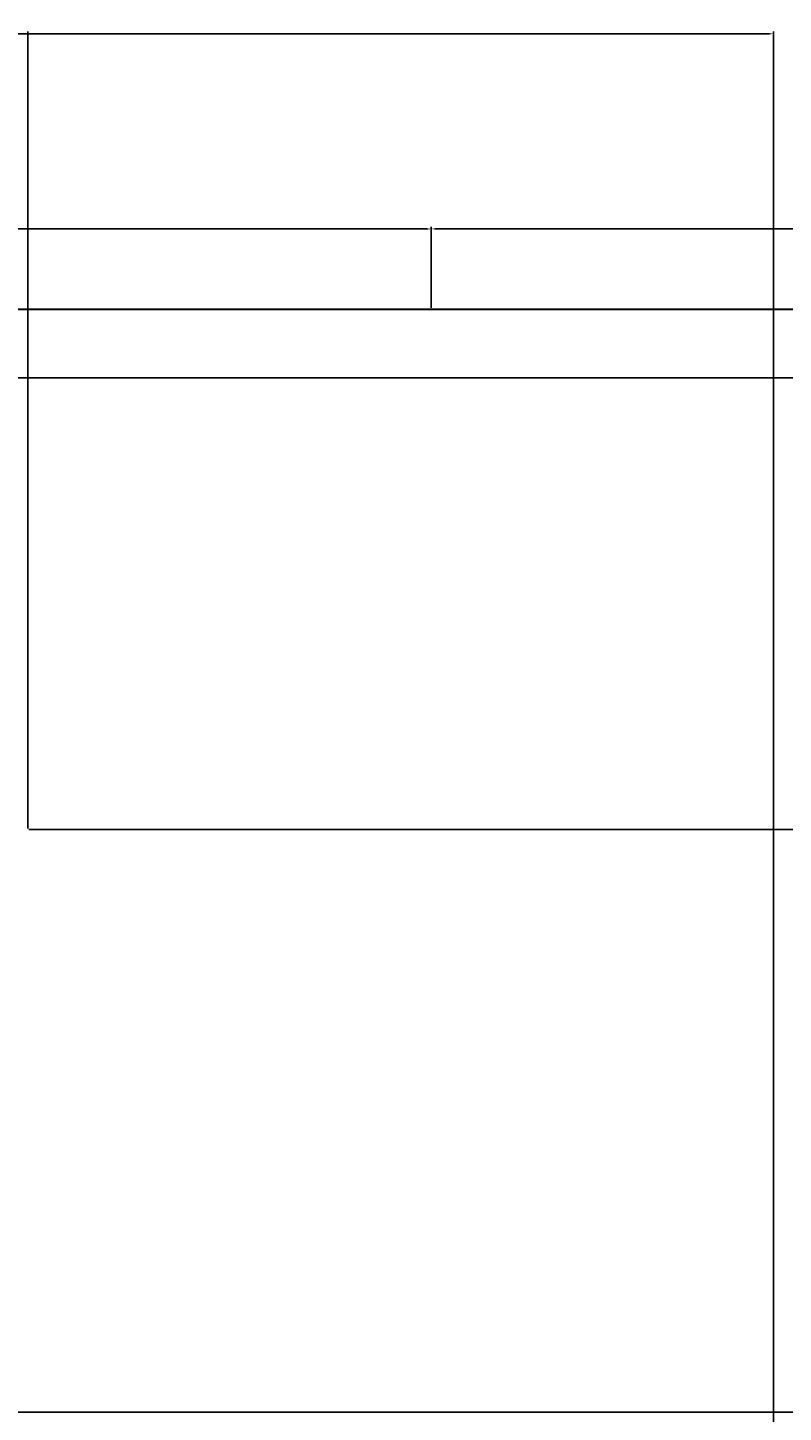
# Model space of a CAD drawing. Units: millimetres. Extents: x 2332 to 5836, y -853 to 2199.
# Tile 13 of 16: x 4341 to 4779, y 1368 to 2171. Entities that reach past the tile are written whole.
import ezdxf

# ---------------------------------------------------------------- set-up
doc = ezdxf.new("R2010")
doc.units = ezdxf.units.MM
for name, color, linetype, lineweight in [('A-ANNO-DIMS', 2, 'Continuous', 18), ('A-WALL', 8, 'Continuous', 30), ('SHELF', 40, 'Continuous', 25)]:
    doc.layers.add(name, color=color, linetype=linetype, lineweight=lineweight)
doc.styles.get("Standard").update_dxf_attribs({"font": 'arial.ttf'})
doc.dimstyles.new('ISO-25', dxfattribs={"dimtxt": 2.5, "dimasz": 2.5, "dimexe": 1.25, "dimexo": 0.625, "dimtad": 1, "dimtxsty": 'Standard', "dimcen": 2.5, "dimadec": 0, "dimazin": 0, "dimtfac": 1, "dimtmove": 0, "dimatfit": 3, "dimfxl": 1, "dimarcsym": 0})

# ---------------------------------------------------------------- blocks, each defined once
blk = doc.blocks.new('*D4')
at = {"layer": 'A-ANNO-DIMS', "color": 0, "lineweight": -2, "transparency": 16777216}
for p, q in [((3635.04, 2008.43), (3635.04, 2055.5)), ((3637.54, 2054.25), (4572.54, 2054.25)), ((4575.04, 2008.43), (4575.04, 2055.5))]:
    blk.add_line(p, q, dxfattribs=at)
at = {"layer": 'A-ANNO-DIMS', "color": 0, "transparency": 16777216}
for points in [[(3637.54, 2054.66), (3637.54, 2053.83), (3635.04, 2054.25)], [(4572.54, 2054.66), (4572.54, 2053.83), (4575.04, 2054.25)]]:
    blk.add_solid(points, dxfattribs=at)
at = {"layer": 'Defpoints', "color": 0, "transparency": 16777216}
for p in [(4575.04, 2054.25), (3635.04, 2007.8), (4575.04, 2007.8)]:
    blk.add_point(p, dxfattribs=at)
at = {"layer": 'A-ANNO-DIMS', "color": 0, "transparency": 16777216, "insert": (4105.04, 2056.15), "char_height": 2.5, "attachment_point": 5}
blk.add_mtext('940', dxfattribs=at)
blk = doc.blocks.new('*D5')
at = {"layer": 'A-ANNO-DIMS', "color": 0, "lineweight": -2, "transparency": 16777216}
for p, q in [((4575.04, 2008.43), (4575.04, 2055.5)), ((4577.54, 2054.25), (5122.54, 2054.25)), ((5125.04, 2008.43), (5125.04, 2055.5))]:
    blk.add_line(p, q, dxfattribs=at)
at = {"layer": 'A-ANNO-DIMS', "color": 0, "transparency": 16777216}
for points in [[(4577.54, 2054.66), (4577.54, 2053.83), (4575.04, 2054.25)], [(5122.54, 2054.66), (5122.54, 2053.83), (5125.04, 2054.25)]]:
    blk.add_solid(points, dxfattribs=at)
at = {"layer": 'Defpoints', "color": 0, "transparency": 16777216}
for p in [(5125.04, 2054.25), (4575.04, 2007.8), (5125.04, 2007.8)]:
    blk.add_point(p, dxfattribs=at)
at = {"layer": 'A-ANNO-DIMS', "color": 0, "transparency": 16777216, "insert": (4850.04, 2056.15), "char_height": 2.5, "attachment_point": 5}
blk.add_mtext('550', dxfattribs=at)
blk = doc.blocks.new('*D23')
at = {"layer": 'A-ANNO-DIMS', "color": 0, "lineweight": -2, "transparency": 16777216}
for p, q in [((3646.47, 1030.43), (3646.47, 2168.7)), ((4773.61, 1030.43), (4773.61, 2168.7)), ((3648.97, 2167.45), (4771.11, 2167.45))]:
    blk.add_line(p, q, dxfattribs=at)
at = {"layer": 'A-ANNO-DIMS', "color": 0, "transparency": 16777216}
for points in [[(3648.97, 2167.87), (3648.97, 2167.04), (3646.47, 2167.45)], [(4771.11, 2167.87), (4771.11, 2167.04), (4773.61, 2167.45)]]:
    blk.add_solid(points, dxfattribs=at)
at = {"layer": 'Defpoints', "color": 0, "transparency": 16777216}
for p in [(4773.61, 2167.45), (3646.47, 1029.8), (4773.61, 1029.8)]:
    blk.add_point(p, dxfattribs=at)
at = {"layer": 'A-ANNO-DIMS', "color": 0, "transparency": 16777216, "insert": (4210.04, 2169.33), "char_height": 2.5, "attachment_point": 5}
blk.add_mtext('1127.1', dxfattribs=at)
blk = doc.blocks.new('*D24')
at = {"layer": 'A-ANNO-DIMS', "color": 0, "lineweight": -2, "transparency": 16777216}
for p, q in [((4079.19, 1706.43), (4079.19, 2168.7)), ((4340.89, 1706.43), (4340.89, 2168.7)), ((4081.69, 2167.45), (4338.39, 2167.45))]:
    blk.add_line(p, q, dxfattribs=at)
at = {"layer": 'A-ANNO-DIMS', "color": 0, "transparency": 16777216}
for points in [[(4081.69, 2167.87), (4081.69, 2167.04), (4079.19, 2167.45)], [(4338.39, 2167.87), (4338.39, 2167.04), (4340.89, 2167.45)]]:
    blk.add_solid(points, dxfattribs=at)
at = {"layer": 'Defpoints', "color": 0, "transparency": 16777216}
for p in [(4340.89, 2167.45), (4079.19, 1705.81), (4340.89, 1705.81)]:
    blk.add_point(p, dxfattribs=at)
at = {"layer": 'A-ANNO-DIMS', "color": 0, "transparency": 16777216, "insert": (4210.04, 2169.35), "char_height": 2.5, "attachment_point": 5}
blk.add_mtext('261.7', dxfattribs=at)
blk = doc.blocks.new('*D25')
at = {"layer": 'A-ANNO-DIMS', "color": 0, "lineweight": -2, "transparency": 16777216}
for p, q in [((4341.52, 1705.81), (5835.94, 1705.81)), ((5834.69, 1032.3), (5834.69, 1703.31)), ((4341.52, 1029.8), (5835.94, 1029.8))]:
    blk.add_line(p, q, dxfattribs=at)
at = {"layer": 'A-ANNO-DIMS', "color": 0, "transparency": 16777216}
for points in [[(5834.27, 1703.31), (5835.11, 1703.31), (5834.69, 1705.81)], [(5834.27, 1032.3), (5835.11, 1032.3), (5834.69, 1029.8)]]:
    blk.add_solid(points, dxfattribs=at)
at = {"layer": 'Defpoints', "color": 0, "transparency": 16777216}
for p in [(4340.89, 1705.81), (5834.69, 1705.81), (4340.89, 1029.8)]:
    blk.add_point(p, dxfattribs=at)
at = {"layer": 'A-ANNO-DIMS', "color": 0, "transparency": 16777216, "insert": (5832.79, 1367.8), "char_height": 2.5, "attachment_point": 5, "rotation": 90}
blk.add_mtext('676', dxfattribs=at)

msp = doc.modelspace()

# ---------------------------------------------------------------- linework, layer by layer
at = {"layer": 'A-WALL'}
for p, q in [((3635.04, 2007.803), (4575.04, 2007.803)), ((4575.04, 2007.803), (5125.04, 2007.803))]:
    msp.add_line(p, q, dxfattribs=at)
at = {"layer": 'SHELF'}
for p, q in [((3095.04, 1967.803), (4785.04, 1967.803)), ((3635.04, 1367.803), (4785.04, 1367.803))]:
    msp.add_line(p, q, dxfattribs=at)

# ---------------------------------------------------------------- dimensions: what is measured, and where the dimension line sits
at = {"layer": 'A-ANNO-DIMS'}
for base, p1, p2, override, picture, middle in [((4773.612, 2167.453), (3646.468, 1029.801), (4773.612, 1029.801), {"dimdec": 1, "dimlfac": 1, "dimrnd": 0, "dimzin": 0, "dimdsep": 46, "dimlunit": 2}, '*D23', (4210.04, 2169.334)), ((4340.894, 2167.453), (4079.186, 1705.805), (4340.894, 1705.805), {"dimdec": 1, "dimlfac": 1, "dimrnd": 0, "dimzin": 0, "dimdsep": 46, "dimlunit": 2}, '*D24', (4210.04, 2169.355)), ((4575.04, 2054.248), (3635.04, 2007.803), (4575.04, 2007.803), {"dimclrd": 0, "dimclre": 0, "dimclrt": 0}, '*D4', (4105.04, 2056.149)), ((5125.04, 2054.248), (4575.04, 2007.803), (5125.04, 2007.803), {"dimclrd": 0, "dimclre": 0, "dimclrt": 0}, '*D5', (4850.04, 2056.149))]:
    dim = msp.add_linear_dim(base=base, p1=p1, p2=p2, dimstyle='ISO-25', override=override, dxfattribs=at)
    dim.commit()
    dim.dimension.update_dxf_attribs({"geometry": picture, "text_midpoint": middle})
dim = msp.add_linear_dim(base=(5834.69, 1705.805), p1=(4340.894, 1029.801), p2=(4340.894, 1705.805), angle=90, dimstyle='ISO-25', override={"dimdec": 0, "dimlfac": 1, "dimrnd": 0, "dimzin": 0, "dimdsep": 46, "dimlunit": 2}, dxfattribs=at)
dim.commit()
dim.dimension.update_dxf_attribs({"geometry": '*D25', "text_midpoint": (5832.788, 1367.803)})

doc.saveas('drawing.dxf')
